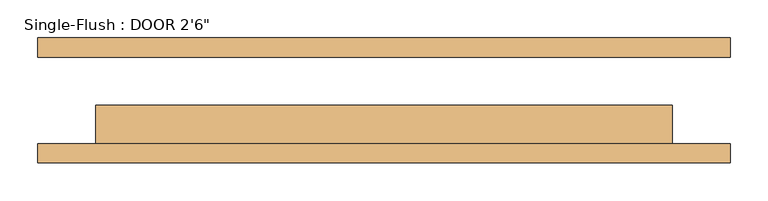
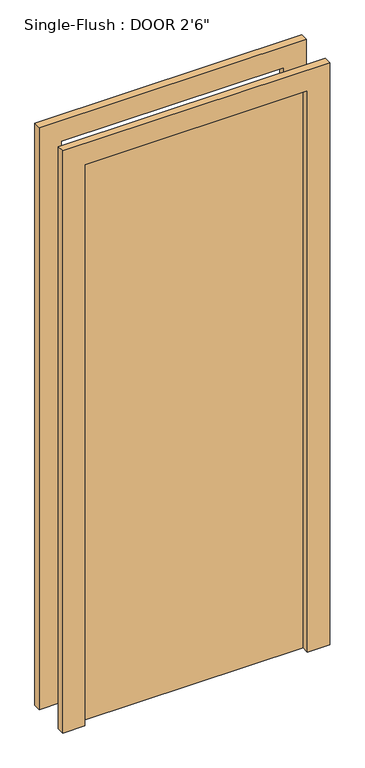
"""IFC4 building model written with IfcOpenShell, lengths in millimetres: door geometry."""

from ifc_helpers import new_model, si_unit, frame, origin, origin_with_axes, place, context, project, spatial, polyline, outline, extrude, source, transform, mapped, element, save


def door_f2b275c1(model_context):
    return source(origin(), model_context, "Body", "SweptSolid", [
        extrude(outline(polyline([(2108.2, -457.2), (0.0, -457.2), (0.0, -381.0), (2032.0, -381.0), (2032.0, 381.0), (0.0, 381.0), (0.0, 457.2), (2108.2, 457.2), (2108.2, -457.2)])), frame((0.0, -82.55, 0.0), z_axis=(0.0, 1.0, 0.0), x_axis=(0.0, 0.0, 1.0)), (0.0, 0.0, 1.0), 25.4),
        extrude(outline(polyline([(2108.2, 457.2), (2108.2, -457.2), (0.0, -457.2), (0.0, -381.0), (2032.0, -381.0), (2032.0, 381.0), (0.0, 381.0), (0.0, 457.2), (2108.2, 457.2)])), frame((0.0, 57.15, 0.0), z_axis=(0.0, 1.0, 0.0), x_axis=(0.0, 0.0, 1.0)), (0.0, 0.0, 1.0), 25.4),
        extrude(outline(polyline([(381.0, -6.35), (381.0, -57.15), (-381.0, -57.15), (-381.0, -6.35), (381.0, -6.35)])), origin_with_axes(), (0.0, 0.0, 1.0), 2032.0),
    ])


if __name__ == "__main__":
    model = new_model("IFC4")
    model_context = context("Model", 3, world=origin())
    ifc_project = project(units=[si_unit("LENGTHUNIT", "METRE", prefix="MILLI")], contexts=[model_context])
    site = spatial("IfcSite", under=ifc_project)
    building = spatial("IfcBuilding", under=site)
    placement = place(None, origin())
    door_shape = door_f2b275c1(model_context)
    element("IfcDoor", 1, ObjectType="Single-Flush : DOOR 2'6\"", at=placement, inside=building, context=model_context, shape_type="MappedRepresentation", body=[
        mapped(door_shape, transform((0.0, 0.0, 0.0), x_axis=(1.0, 0.0, 0.0), y_axis=(0.0, 1.0, 0.0), z_axis=(0.0, 0.0, 1.0))),
    ])
    save(model, "model.ifc")

# Revit data of these elements
# Type "Single-Flush : DOOR 2'6\""
#   Type Mark = "8"
#   Construction Type Id = "MDOOR"
#   Assembly Code = "C1020"
#   Analytic Construction = "Metal"
#   Thickness = 0' - 2"
#   Heat Transfer Coefficient (U) = 0.651978 BTU/(h·ft²·°F)
#   Height = 6' - 8"
#   Trim Projection Ext = 0' - 1"
#   Trim Projection Int = 0' - 1"
#   Trim Width = 0' - 3"
#   Width = 2' - 6"
#   Define Thermal Properties by = 1
#   Door Material = Door - Panel
#   Frame Material = Door - Frame
#   Visual Light Transmittance = 0
#   Solar Heat Gain Coefficient = 0
#   Function = (empty or 0)
#   Wall Closure = (empty or 0)
# Element 1 (IfcDoor, "Single-Flush : DOOR 2'6\"")
#   Materials on its faces: "Door - Frame", "Door - Panel"
# Materials
#   "Door - Panel": class "Wood", colour RGB 210 159 95, transparency 0, Cost = 0
#   "Door - Frame": colour RGB 118 70 51, transparency 0, Cost = 0
